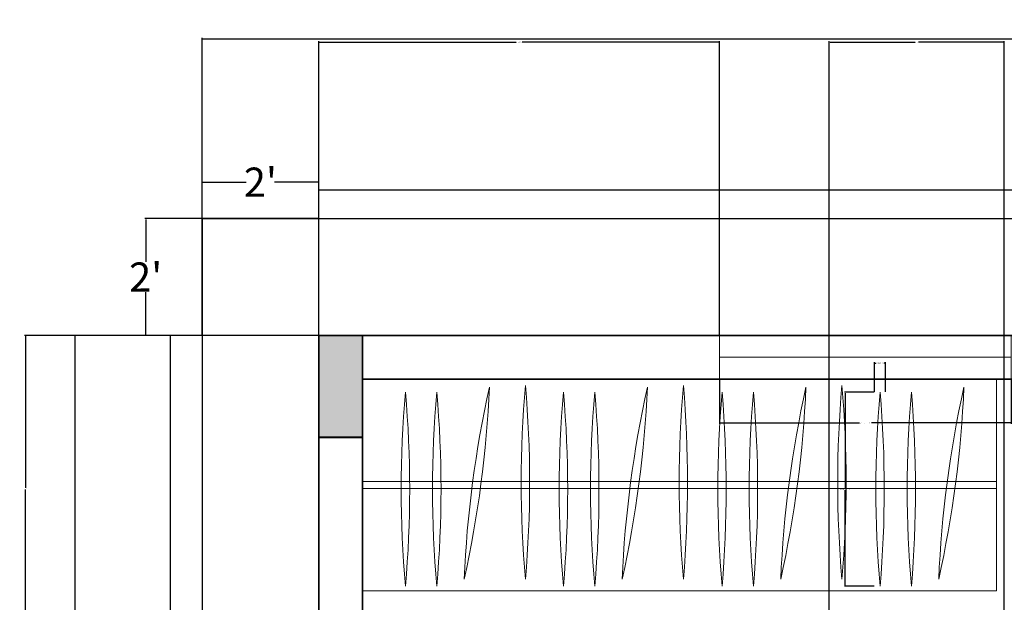
# Model space of a CAD drawing. Units: inches. Extents: x -36 to 401, y -686 to 73.
# Tile 13 of 15: x -36 to 167, y -47 to 73. Entities that reach past the tile are written whole.
import ezdxf

# ---------------------------------------------------------------- set-up
doc = ezdxf.new("R2010")
doc.units = ezdxf.units.IN
doc.header["$MEASUREMENT"] = 0
for name, color, linetype, lineweight in [('A-ANNO-DIMS', 2, 'Continuous', 18), ('A-COLS', 7, 'Continuous', 40), ('A-COLS-PATT', 22, 'Continuous', 13), ('A-FLOR-CASE', 9, 'Continuous', 18), ('A-GLAZ', 4, 'Continuous', 18), ('A-WALL', 7, 'Continuous', 35), ('C-PROP', 7, 'Continuous', 25)]:
    doc.layers.add(name, color=color, linetype=linetype, lineweight=lineweight)
doc.styles.get("Standard").update_dxf_attribs({"font": 'arial.ttf'})
doc.dimstyles.get("Standard").update_dxf_attribs({"dimtxt": 0.18, "dimasz": 0.18, "dimexe": 0.18, "dimexo": 0.0625, "dimgap": 0.09, "dimtad": 0, "dimtih": 1, "dimtoh": 1, "dimdec": 0, "dimzin": 0, "dimdsep": 46, "dimlunit": 3, "dimtxsty": 'Standard', "dimcen": 0.09, "dimadec": 0, "dimazin": 0, "dimtfac": 1, "dimtdec": 0, "dimtofl": 0, "dimtmove": 0, "dimatfit": 3, "dimfxl": 1, "dimtolj": 1, "dimtzin": 0, "dimarcsym": 0})

# ---------------------------------------------------------------- blocks, each defined once
blk = doc.blocks.new('*D4')
at = {"layer": 'A-ANNO-DIMS', "color": 0, "lineweight": -2, "transparency": 16777216}
for p, q in [((1.69, 7.85), (1.69, 39.47)), ((1.87, 39.29), (10.79, 39.29)), ((25.51, 39.29), (16.59, 39.29)), ((25.69, 7.85), (25.69, 39.47))]:
    blk.add_line(p, q, dxfattribs=at)
at = {"layer": 'A-ANNO-DIMS', "color": 0, "transparency": 16777216}
for points in [[(1.87, 39.32), (1.87, 39.26), (1.69, 39.29)], [(25.51, 39.32), (25.51, 39.26), (25.69, 39.29)]]:
    blk.add_solid(points, dxfattribs=at)
at = {"layer": 'Defpoints', "color": 0, "transparency": 16777216}
for p in [(1.69, 39.29), (1.69, 7.79), (25.69, 7.79)]:
    blk.add_point(p, dxfattribs=at)
at = {"layer": 'A-ANNO-DIMS', "color": 0, "transparency": 16777216, "insert": (13.69, 39.29), "char_height": 6, "attachment_point": 5}
blk.add_mtext("\\A1;2'", dxfattribs=at)
blk = doc.blocks.new('*D5')
at = {"layer": 'A-ANNO-DIMS', "color": 0, "lineweight": -2, "transparency": 16777216}
for p, q in [((25.69, 7.85), (25.69, 37.9)), ((25.87, 37.72), (181.74, 37.72)), ((358.51, 37.72), (202.64, 37.72)), ((358.69, 7.85), (358.69, 37.9))]:
    blk.add_line(p, q, dxfattribs=at)
at = {"layer": 'A-ANNO-DIMS', "color": 0, "transparency": 16777216}
for points in [[(25.87, 37.75), (25.87, 37.69), (25.69, 37.72)], [(358.51, 37.75), (358.51, 37.69), (358.69, 37.72)]]:
    blk.add_solid(points, dxfattribs=at)
at = {"layer": 'Defpoints', "color": 0, "transparency": 16777216}
for p in [(358.69, 37.72), (25.69, 7.79), (358.69, 7.79)]:
    blk.add_point(p, dxfattribs=at)
at = {"layer": 'A-ANNO-DIMS', "color": 0, "transparency": 16777216, "insert": (192.19, 37.72), "char_height": 6, "attachment_point": 5}
blk.add_mtext('\\A1;27\'-9"', dxfattribs=at)
blk = doc.blocks.new('*D8')
at = {"layer": 'A-ANNO-DIMS', "color": 0, "lineweight": -2, "transparency": 16777216}
for p, q in [((25.63, 7.79), (-24.68, 7.79)), ((-24.5, 7.61), (-24.5, -317.56)), ((-24.5, -649.03), (-24.5, -323.86)), ((1.63, -649.21), (-24.68, -649.21))]:
    blk.add_line(p, q, dxfattribs=at)
at = {"layer": 'A-ANNO-DIMS', "color": 0, "transparency": 16777216}
for points in [[(-24.53, 7.61), (-24.47, 7.61), (-24.5, 7.79)], [(-24.53, -649.03), (-24.47, -649.03), (-24.5, -649.21)]]:
    blk.add_solid(points, dxfattribs=at)
at = {"layer": 'Defpoints', "color": 0, "transparency": 16777216}
for p in [(25.69, 7.79), (-24.5, -649.21), (1.69, -649.21)]:
    blk.add_point(p, dxfattribs=at)
at = {"layer": 'A-ANNO-DIMS', "color": 0, "transparency": 16777216, "insert": (-24.5, -320.71), "char_height": 6, "attachment_point": 5}
blk.add_mtext('\\A1;54\'-9"', dxfattribs=at)
blk = doc.blocks.new('*D9')
at = {"layer": 'A-ANNO-DIMS', "color": 0, "lineweight": -2, "transparency": 16777216}
for p, q in [((1.69, 31.85), (1.69, 68.93)), ((364.69, 31.85), (364.69, 68.93)), ((1.87, 68.75), (172.79, 68.75)), ((364.51, 68.75), (193.58, 68.75))]:
    blk.add_line(p, q, dxfattribs=at)
at = {"layer": 'A-ANNO-DIMS', "color": 0, "transparency": 16777216}
for points in [[(1.87, 68.78), (1.87, 68.72), (1.69, 68.75)], [(364.51, 68.78), (364.51, 68.72), (364.69, 68.75)]]:
    blk.add_solid(points, dxfattribs=at)
at = {"layer": 'Defpoints', "color": 0, "transparency": 16777216}
for p in [(364.69, 68.75), (1.69, 31.79), (364.69, 31.79)]:
    blk.add_point(p, dxfattribs=at)
at = {"layer": 'A-ANNO-DIMS', "color": 0, "transparency": 16777216, "insert": (183.19, 68.75), "char_height": 6, "attachment_point": 5}
blk.add_mtext('\\A1;30\'-3"', dxfattribs=at)
blk = doc.blocks.new('*D10')
at = {"layer": 'A-ANNO-DIMS', "color": 0, "lineweight": -2, "transparency": 16777216}
for p, q in [((25.63, 31.79), (-10.08, 31.79)), ((-9.9, 31.61), (-9.9, 22.89)), ((-9.9, 7.97), (-9.9, 16.69)), ((25.63, 7.79), (-10.08, 7.79))]:
    blk.add_line(p, q, dxfattribs=at)
at = {"layer": 'A-ANNO-DIMS', "color": 0, "transparency": 16777216}
for points in [[(-9.93, 31.61), (-9.87, 31.61), (-9.9, 31.79)], [(-9.93, 7.97), (-9.87, 7.97), (-9.9, 7.79)]]:
    blk.add_solid(points, dxfattribs=at)
at = {"layer": 'Defpoints', "color": 0, "transparency": 16777216}
for p in [(-9.9, 31.79), (25.69, 31.79), (25.69, 7.79)]:
    blk.add_point(p, dxfattribs=at)
at = {"layer": 'A-ANNO-DIMS', "color": 0, "transparency": 16777216, "insert": (-9.9, 19.79), "char_height": 6, "attachment_point": 5}
blk.add_mtext("\\A1;2'", dxfattribs=at)
blk = doc.blocks.new('*D11')
at = {"layer": 'A-ANNO-DIMS', "color": 0, "lineweight": -2, "transparency": 16777216}
for p, q in [((25.63, 7.79), (-5.02, 7.79)), ((-4.84, 7.61), (-4.84, -268.06)), ((-4.84, -550.03), (-4.84, -274.36)), ((25.63, -550.21), (-5.02, -550.21))]:
    blk.add_line(p, q, dxfattribs=at)
at = {"layer": 'A-ANNO-DIMS', "color": 0, "transparency": 16777216}
for points in [[(-4.87, 7.61), (-4.81, 7.61), (-4.84, 7.79)], [(-4.87, -550.03), (-4.81, -550.03), (-4.84, -550.21)]]:
    blk.add_solid(points, dxfattribs=at)
at = {"layer": 'Defpoints', "color": 0, "transparency": 16777216}
for p in [(25.69, 7.79), (-4.84, -550.21), (25.69, -550.21)]:
    blk.add_point(p, dxfattribs=at)
at = {"layer": 'A-ANNO-DIMS', "color": 0, "transparency": 16777216, "insert": (-4.84, -271.21), "char_height": 6, "attachment_point": 5}
blk.add_mtext('\\A1;46\'-6"', dxfattribs=at)
blk = doc.blocks.new('WIN-60IN')
for p, q in [((0, 9), (60, 9)), ((0, 0), (0, 9)), ((60, 9), (60, 0)), ((0, 4.5), (60, 4.5)), ((60, 0), (0, 0))]:
    blk.add_line(p, q)
blk = doc.blocks.new('GARMENT-ON-RAIL-LARGE')
for centre, start, end in [((228.72, 19.92), 175.0028, 184.9972), ((-226.98, 19.92), 355.0028, 4.9972)]:
    blk.add_arc(centre, 228.72, start, end)
blk = doc.blocks.new('*D29')
at = {"layer": 'A-ANNO-DIMS', "color": 0, "lineweight": -2, "transparency": 16777216}
for p, q in [((139.9, -3.89), (133.81, -3.89)), ((133.99, -4.07), (133.99, -23.63)), ((133.99, -43.56), (133.99, -24)), ((139.9, -43.74), (133.81, -43.74))]:
    blk.add_line(p, q, dxfattribs=at)
at = {"layer": 'A-ANNO-DIMS', "color": 0, "transparency": 16777216}
for points in [[(133.96, -4.07), (134.02, -4.07), (133.99, -3.89)], [(133.96, -43.56), (134.02, -43.56), (133.99, -43.74)]]:
    blk.add_solid(points, dxfattribs=at)
at = {"layer": 'Defpoints', "color": 0, "transparency": 16777216}
for p in [(133.99, -3.89), (139.97, -3.89), (139.97, -43.74)]:
    blk.add_point(p, dxfattribs=at)
at = {"layer": 'A-ANNO-DIMS', "color": 0, "transparency": 16777216, "insert": (133.99, -23.81), "char_height": 0.18, "attachment_point": 5}
blk.add_mtext('\\A1;HANGER 3\'-4" TYP.', dxfattribs=at)
blk = doc.blocks.new('*D30')
at = {"layer": 'A-ANNO-DIMS', "color": 0, "lineweight": -2, "transparency": 16777216}
for p, q in [((139.97, -3.83), (139.97, 2.27)), ((140.15, 2.09), (140.28, 2.09)), ((142.1, 2.09), (141.97, 2.09)), ((142.28, -3.83), (142.28, 2.27))]:
    blk.add_line(p, q, dxfattribs=at)
at = {"layer": 'A-ANNO-DIMS', "color": 0, "transparency": 16777216}
for points in [[(140.15, 2.12), (140.15, 2.06), (139.97, 2.09)], [(142.1, 2.12), (142.1, 2.06), (142.28, 2.09)]]:
    blk.add_solid(points, dxfattribs=at)
at = {"layer": 'Defpoints', "color": 0, "transparency": 16777216}
for p in [(142.28, 2.09), (139.97, -3.89), (142.28, -3.89)]:
    blk.add_point(p, dxfattribs=at)
at = {"layer": 'A-ANNO-DIMS', "color": 0, "transparency": 16777216, "insert": (141.12, 2.09), "char_height": 0.18, "attachment_point": 5}
blk.add_mtext('\\A1;0\'-2 1/2" TYP.', dxfattribs=at)
blk = doc.blocks.new('*D37')
at = {"layer": 'A-ANNO-DIMS', "color": 0, "lineweight": -2, "transparency": 16777216}
for p, q in [((108.13, -1.27), (108.13, -10.39)), ((168.13, -1.27), (168.13, -10.39)), ((108.31, -10.21), (136.9, -10.21)), ((167.95, -10.21), (139.35, -10.21))]:
    blk.add_line(p, q, dxfattribs=at)
at = {"layer": 'A-ANNO-DIMS', "color": 0, "transparency": 16777216}
for points in [[(108.31, -10.18), (108.31, -10.24), (108.13, -10.21)], [(167.95, -10.18), (167.95, -10.24), (168.13, -10.21)]]:
    blk.add_solid(points, dxfattribs=at)
at = {"layer": 'Defpoints', "color": 0, "transparency": 16777216}
for p in [(108.13, -1.21), (168.13, -1.21), (168.13, -10.21)]:
    blk.add_point(p, dxfattribs=at)
at = {"layer": 'A-ANNO-DIMS', "color": 0, "transparency": 16777216, "insert": (138.13, -10.21), "char_height": 0.18, "attachment_point": 5}
blk.add_mtext('\\A1;WINDOW 5\'-0" TYP.', dxfattribs=at)
blk = doc.blocks.new('*D66')
at = {"layer": 'A-ANNO-DIMS', "color": 0, "lineweight": -2, "transparency": 16777216}
for p, q in [((25.69, 7.85), (25.69, 68.27)), ((25.87, 68.09), (66.3, 68.09)), ((107.95, 68.09), (67.52, 68.09)), ((108.13, 7.85), (108.13, 68.27))]:
    blk.add_line(p, q, dxfattribs=at)
at = {"layer": 'A-ANNO-DIMS', "color": 0, "transparency": 16777216}
for points in [[(25.87, 68.12), (25.87, 68.06), (25.69, 68.09)], [(107.95, 68.12), (107.95, 68.06), (108.13, 68.09)]]:
    blk.add_solid(points, dxfattribs=at)
at = {"layer": 'Defpoints', "color": 0, "transparency": 16777216}
for p in [(108.13, 68.09), (25.69, 7.79), (108.13, 7.79)]:
    blk.add_point(p, dxfattribs=at)
at = {"layer": 'A-ANNO-DIMS', "color": 0, "transparency": 16777216, "insert": (66.91, 68.09), "char_height": 0.18, "attachment_point": 5}
blk.add_mtext('\\A1;6\'-10 1/2"', dxfattribs=at)
blk = doc.blocks.new('*D68')
at = {"layer": 'A-ANNO-DIMS', "color": 0, "lineweight": -2, "transparency": 16777216}
for p, q in [((25.63, 7.79), (-34.79, 7.79)), ((-34.61, 7.61), (-34.61, -23.53)), ((-34.61, -55.03), (-34.61, -23.89)), ((25.63, -55.21), (-34.79, -55.21))]:
    blk.add_line(p, q, dxfattribs=at)
at = {"layer": 'A-ANNO-DIMS', "color": 0, "transparency": 16777216}
for points in [[(-34.64, 7.61), (-34.58, 7.61), (-34.61, 7.79)], [(-34.64, -55.03), (-34.58, -55.03), (-34.61, -55.21)]]:
    blk.add_solid(points, dxfattribs=at)
at = {"layer": 'Defpoints', "color": 0, "transparency": 16777216}
for p in [(25.69, 7.79), (-34.61, -55.21), (25.69, -55.21)]:
    blk.add_point(p, dxfattribs=at)
at = {"layer": 'A-ANNO-DIMS', "color": 0, "transparency": 16777216, "insert": (-34.61, -23.71), "char_height": 0.18, "attachment_point": 5}
blk.add_mtext('\\A1;5\'-3"', dxfattribs=at)
blk = doc.blocks.new('*D79')
at = {"layer": 'A-ANNO-DIMS', "color": 0, "lineweight": -2, "transparency": 16777216}
for p, q in [((130.69, -398.65), (130.69, 68.27)), ((130.87, 68.09), (148.36, 68.09)), ((166.51, 68.09), (149.02, 68.09)), ((166.69, -398.65), (166.69, 68.27))]:
    blk.add_line(p, q, dxfattribs=at)
at = {"layer": 'A-ANNO-DIMS', "color": 0, "transparency": 16777216}
for points in [[(130.87, 68.12), (130.87, 68.06), (130.69, 68.09)], [(166.51, 68.12), (166.51, 68.06), (166.69, 68.09)]]:
    blk.add_solid(points, dxfattribs=at)
at = {"layer": 'Defpoints', "color": 0, "transparency": 16777216}
for p in [(166.69, 68.09), (130.69, -398.71), (166.69, -398.71)]:
    blk.add_point(p, dxfattribs=at)
at = {"layer": 'A-ANNO-DIMS', "color": 0, "transparency": 16777216, "insert": (148.69, 68.09), "char_height": 0.18, "attachment_point": 5}
blk.add_mtext('\\A1;3\'-0"', dxfattribs=at)

msp = doc.modelspace()

# ---------------------------------------------------------------- hatches: boundary and pattern name
at = {"layer": 'A-COLS-PATT'}
h = msp.add_hatch(color=256, dxfattribs=at)
h.dxf.hatch_style = 1
h.paths.add_polyline_path([(34.69, 7.79), (25.69, 7.79), (25.69, -13.21), (34.69, -13.21)])
h.paths.add_polyline_path([(172.69, -13.21), (177.19, -13.21), (181.69, -13.21), (181.69, 7.79), (172.69, 7.79)])
h.paths.add_polyline_path([(322.69, 7.79), (313.69, 7.79), (313.69, -13.21), (322.69, -13.21)])
h.paths.add_polyline_path([(322.69, -157.21), (313.69, -157.21), (313.69, -178.21), (322.69, -178.21)])
h.paths.add_polyline_path([(172.69, -178.21), (177.19, -178.21), (181.69, -178.21), (181.69, -157.21), (177.19, -157.21), (172.69, -157.21)])
h.paths.add_polyline_path([(25.69, -178.21), (34.69, -178.21), (34.69, -157.21), (25.69, -157.21)])
h.paths.add_polyline_path([(34.69, -325.21), (25.69, -325.21), (25.69, -346.21), (34.69, -346.21)])
h.paths.add_polyline_path([(181.69, -325.21), (177.19, -325.21), (172.69, -325.21), (172.69, -346.21), (177.19, -346.21), (181.69, -346.21)])
h.paths.add_polyline_path([(322.69, -325.21), (313.69, -325.21), (313.69, -346.21), (322.69, -346.21)])
h.paths.add_polyline_path([(364.69, -451.21), (358.69, -451.21), (358.69, -472.21), (364.69, -472.21)])
h.paths.add_polyline_path([(181.69, -451.21), (177.19, -451.21), (172.69, -451.21), (172.69, -472.21), (177.19, -472.21), (181.69, -472.21)])
h.paths.add_polyline_path([(25.69, -472.21), (34.69, -472.21), (34.69, -451.21), (25.69, -451.21)])

# ---------------------------------------------------------------- linework, layer by layer
at = {"layer": 'A-COLS'}
msp.add_line((34.69, -13.21), (25.69, -13.21), dxfattribs=at)
at = {"layer": 'A-FLOR-CASE'}
for p, q in [((165.09, -1.21), (34.69, -1.21)), ((34.69, -1.21), (34.69, -44.68)), ((165.09, -1.21), (165.09, -44.68)), ((165.09, -22.22), (34.69, -22.22)), ((165.09, -23.67), (34.69, -23.67)), ((165.09, -44.68), (34.69, -44.68))]:
    msp.add_line(p, q, dxfattribs=at)
at = {"layer": 'A-WALL'}
for p, q in [((25.69, 7.79), (25.69, -178.21)), ((25.69, 7.79), (364.69, 7.79)), ((34.69, 7.79), (34.69, -178.21)), ((34.69, -1.21), (172.69, -1.21))]:
    msp.add_line(p, q, dxfattribs=at)
at = {"layer": 'C-PROP'}
for q in [(1.69, -649.21), (364.69, 31.79)]:
    msp.add_line((1.69, 31.79), q, dxfattribs=at)

# ---------------------------------------------------------------- block references
at = {"layer": 'A-FLOR-CASE'}
for p in [(42.66, -43.74), (49.1, -43.74), (67.32, -42.33), (75.15, -43.74), (81.59, -43.74), (99.81, -42.33), (107.76, -43.74), (114.21, -43.74), (140.26, -43.74), (146.7, -43.74)]:
    msp.add_blockref('GARMENT-ON-RAIL-LARGE', p, dxfattribs=at)
for p, rotation in [((61.66, -2.95), 172.5051423894907), ((94.15, -2.95), 172.5051423894907), ((119.84, -42.23), 352.5051423895281), ((134.16, -2.49), 180), ((152.33, -42.23), 352.5051423896664)]:
    msp.add_blockref('GARMENT-ON-RAIL-LARGE', p, dxfattribs=dict(at, rotation=rotation))
at = {"layer": 'A-GLAZ'}
msp.add_blockref('WIN-60IN', (108.12, -1.21), dxfattribs=at)

# ---------------------------------------------------------------- dimensions: what is measured, and where the dimension line sits
at = {"layer": 'A-ANNO-DIMS'}
for base, p1, p2, override, picture, middle in [((364.69, 68.75), (1.69, 31.79), (364.69, 31.79), {"dimtxt": 6, "dimclrd": 0, "dimclre": 0, "dimclrt": 0}, '*D9', (183.19, 68.75)), ((108.13, 68.09), (25.69, 7.79), (108.13, 7.79), {"dimdec": 1, "dimlfac": 1, "dimrnd": 0, "dimzin": 1, "dimdsep": 46, "dimlunit": 4, "dimfrac": 2}, '*D66', (66.91, 68.09)), ((166.69, 68.09), (130.69, -398.71), (166.69, -398.71), {"dimdec": 1, "dimlfac": 1, "dimrnd": 0, "dimzin": 1, "dimdsep": 46, "dimlunit": 4, "dimfrac": 2}, '*D79', (148.69, 68.09)), ((1.69, 39.29), (25.69, 7.79), (1.69, 7.79), {"dimtxt": 6, "dimclrd": 0, "dimclre": 0, "dimclrt": 0}, '*D4', (13.69, 39.29)), ((358.69, 37.72), (25.69, 7.79), (358.69, 7.79), {"dimtxt": 6, "dimclrd": 0, "dimclre": 0, "dimclrt": 0}, '*D5', (192.19, 37.72))]:
    dim = msp.add_linear_dim(base=base, p1=p1, p2=p2, dimstyle='Standard', override=override, dxfattribs=at)
    dim.commit()
    dim.dimension.update_dxf_attribs({"geometry": picture, "text_midpoint": middle})
for base, p2, override, picture, middle in [((-9.9, 31.79), (25.69, 31.79), {"dimtxt": 6, "dimclrd": 0, "dimclre": 0, "dimclrt": 0}, '*D10', (-9.9, 19.79)), ((-24.5, -649.21), (1.69, -649.21), {"dimtxt": 6, "dimclrd": 0, "dimclre": 0, "dimclrt": 0}, '*D8', (-24.5, -320.71)), ((-34.61, -55.21), (25.69, -55.21), {"dimdec": 1, "dimlfac": 1, "dimrnd": 0, "dimzin": 1, "dimdsep": 46, "dimlunit": 4, "dimfrac": 2}, '*D68', (-34.61, -23.71)), ((-4.84, -550.21), (25.69, -550.21), {"dimtxt": 6, "dimclrd": 0, "dimclre": 0, "dimclrt": 0}, '*D11', (-4.84, -271.21))]:
    dim = msp.add_linear_dim(base=base, p1=(25.69, 7.79), p2=p2, angle=90, dimstyle='Standard', override=override, dxfattribs=at)
    dim.commit()
    dim.dimension.update_dxf_attribs({"geometry": picture, "text_midpoint": middle})
for base, p1, p2, text, picture, middle in [((142.28, 2.09), (139.97, -3.89), (142.28, -3.89), '<> TYP.', '*D30', (141.12, 2.09)), ((168.13, -10.21), (108.13, -1.21), (168.13, -1.21), 'WINDOW <> TYP.', '*D37', (138.13, -10.21))]:
    dim = msp.add_linear_dim(base=base, p1=p1, p2=p2, text=text, dimstyle='Standard', override={"dimdec": 1, "dimlfac": 1, "dimrnd": 0, "dimzin": 1, "dimdsep": 46, "dimlunit": 4, "dimfrac": 2}, dxfattribs=at)
    dim.commit()
    dim.dimension.update_dxf_attribs({"geometry": picture, "text_midpoint": middle})
dim = msp.add_linear_dim(base=(133.9888, -3.8901), p1=(139.9658, -43.7365), p2=(139.9658, -3.8901), angle=90, text='HANGER <> TYP.', dimstyle='Standard', override={"dimdec": 1, "dimlfac": 1, "dimrnd": 0, "dimzin": 1, "dimdsep": 46, "dimlunit": 4, "dimfrac": 2}, dxfattribs=at)
dim.commit()
dim.dimension.update_dxf_attribs({"geometry": '*D29', "text_midpoint": (133.9888, -23.8133)})

doc.saveas('drawing.dxf')
